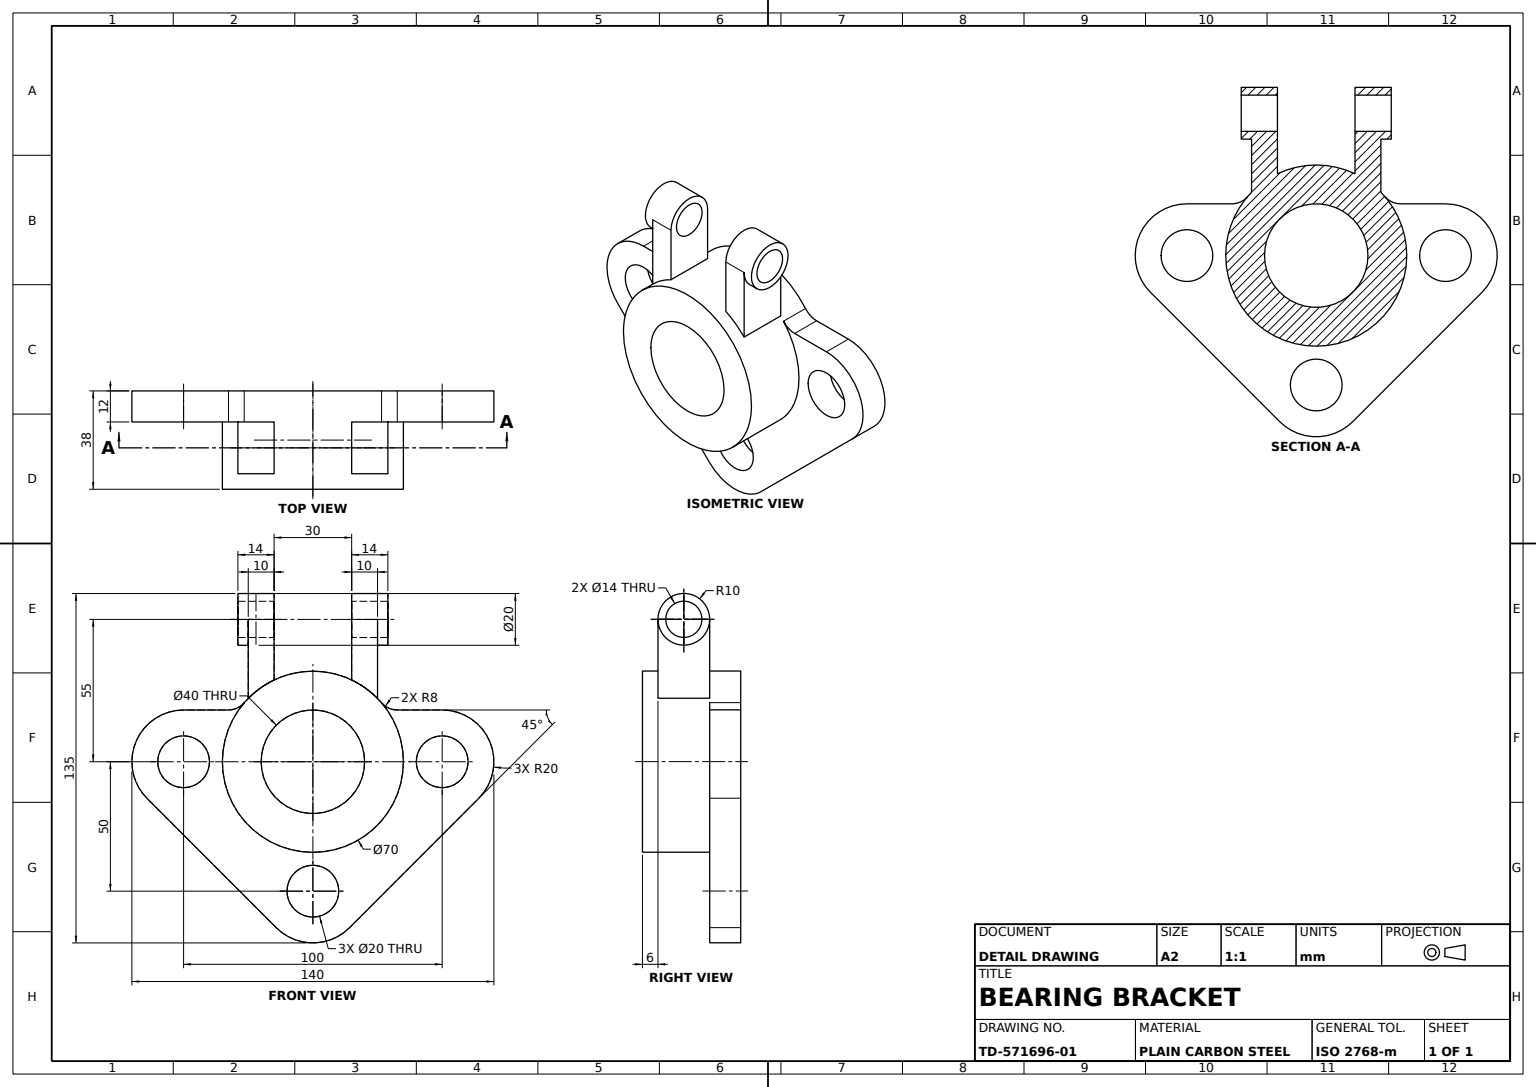
from build123d import *
from build123d.topology import SkipClean

# Parameters (mm, degrees)
HUB_PROFILE_SKETCH_R     = 35
HUB_PROFILE_SKETCH_R_2   = 20
HUB_70_BORE_40_DEPTH     = 38
MOUNTING_FLANGE_SKETCH_R = 10
MOUNTING_FLANGE_DEPTH    = 12
FLANGE_HUB_FILLET_R8_R   = 8
CLEVIS_LUG_SKETCH_W      = 10
CLEVIS_LUG_SKETCH_H      = 20
CLEVIS_LUGS_DEPTH        = 32
LUG_BOSS_SKETCH_A_R      = 10
LUG_BOSS_SKETCH_A_R_2    = 7
LUG_BOSS_A_20_DEPTH      = 14
PIN_START                = -50
PIN_HOLE_SKETCH_R        = 7
PIN_HOLE_14_DEPTH        = 50
LUG_START                = -14
LUG_BOSS_SKETCH_B_R      = 10
LUG_BOSS_SKETCH_B_R_2    = 7
LUG_BOSS_B_20_DEPTH      = 14


with BuildPart() as part:
    # Hub Profile Sketch → Hub Ø70 Bore Ø40 (new body)
    with BuildSketch(Plane.XY):
        Circle(HUB_PROFILE_SKETCH_R)
        Circle(HUB_PROFILE_SKETCH_R_2, mode=Mode.SUBTRACT)
    extrude(amount=HUB_70_BORE_40_DEPTH)

    # Mounting Flange Sketch → Mounting Flange (add)
    with BuildSketch(Plane.XY):
        with BuildLine():
            Line((50, 20), (28.722813233, 20))
            ThreePointArc((28.722813233, 20), (0, -35), (-28.722813233, 20))
            Line((-28.722813233, 20), (-50, 20))
            ThreePointArc((-50, 20), (-68.47759065, 7.653668647), (-64.142135624, -14.142135624))
            Line((-64.142135624, -14.142135624), (-14.142135624, -64.142135624))
            ThreePointArc((-14.142135624, -64.142135624), (0, -70), (14.142135624, -64.142135624))
            Line((14.142135624, -64.142135624), (64.142135624, -14.142135624))
            ThreePointArc((64.142135624, -14.142135624), (68.47759065, 7.653668647), (50, 20))
        make_face()
        with Locations((50, 0)):
            Circle(MOUNTING_FLANGE_SKETCH_R, mode=Mode.SUBTRACT)
        with Locations((0, -50)):
            Circle(MOUNTING_FLANGE_SKETCH_R, mode=Mode.SUBTRACT)
        with Locations(Location((-50, 0, 0), (0, 0, 180))):
            Circle(MOUNTING_FLANGE_SKETCH_R, mode=Mode.SUBTRACT)
    extrude(amount=MOUNTING_FLANGE_DEPTH)

    # Flange Hub Fillet R8
    flange_hub_fillet_r8_edges = [part.edges().sort_by_distance(p)[0] for p in [
        (28.722813233, 20, 6),
        (-28.722813233, 20, 6),
    ]]
    fillet(flange_hub_fillet_r8_edges, radius=FLANGE_HUB_FILLET_R8_R)

    # Clevis Lug Sketch → Clevis Lugs (add)
    with BuildSketch(Plane(origin=(0, 55, 0), x_dir=(1, 0, 0), z_dir=(0, 1, 0))):
        with Locations((-20, -22)):
            Rectangle(CLEVIS_LUG_SKETCH_W, CLEVIS_LUG_SKETCH_H)
        with Locations((20, -22)):
            Rectangle(CLEVIS_LUG_SKETCH_W, CLEVIS_LUG_SKETCH_H)
    extrude(amount=-CLEVIS_LUGS_DEPTH)

    # Lug Boss Sketch A → Lug Boss A Ø20 (add)
    with BuildSketch(Plane.ZY.offset(-15)):
        with Locations((22, 55)):
            Circle(LUG_BOSS_SKETCH_A_R)
        with Locations((22, 55)):
            Circle(LUG_BOSS_SKETCH_A_R_2, mode=Mode.SUBTRACT)
    extrude(amount=-LUG_BOSS_A_20_DEPTH)

    # Pin Hole Sketch → Pin Hole Ø14 (cut)
    with SkipClean():  # the faces are left unmerged after this step: merging them gives an invalid solid
        with BuildSketch(Plane(origin=(25, 0, 0), x_dir=(0, 0, -1), z_dir=(1, 0, 0)).offset(PIN_START)):
            with Locations(Location((-22, 55, 0), (0, 0, 180))):
                Circle(PIN_HOLE_SKETCH_R)
        extrude(amount=PIN_HOLE_14_DEPTH, mode=Mode.SUBTRACT)

    # Lug Boss Sketch B → Lug Boss B Ø20 (add)
    with SkipClean():  # the faces are left unmerged after this step: merging them gives an invalid solid
        with BuildSketch(Plane(origin=(-15, 0, 0), x_dir=(0, 0, -1), z_dir=(1, 0, 0)).offset(LUG_START)):
            with Locations(Location((-22, 55, 0), (0, 0, 180))):
                Circle(LUG_BOSS_SKETCH_B_R)
            with Locations(Location((-22, 55, 0), (0, 0, 180))):
                Circle(LUG_BOSS_SKETCH_B_R_2, mode=Mode.SUBTRACT)
        extrude(amount=LUG_BOSS_B_20_DEPTH)


solid = part.part
